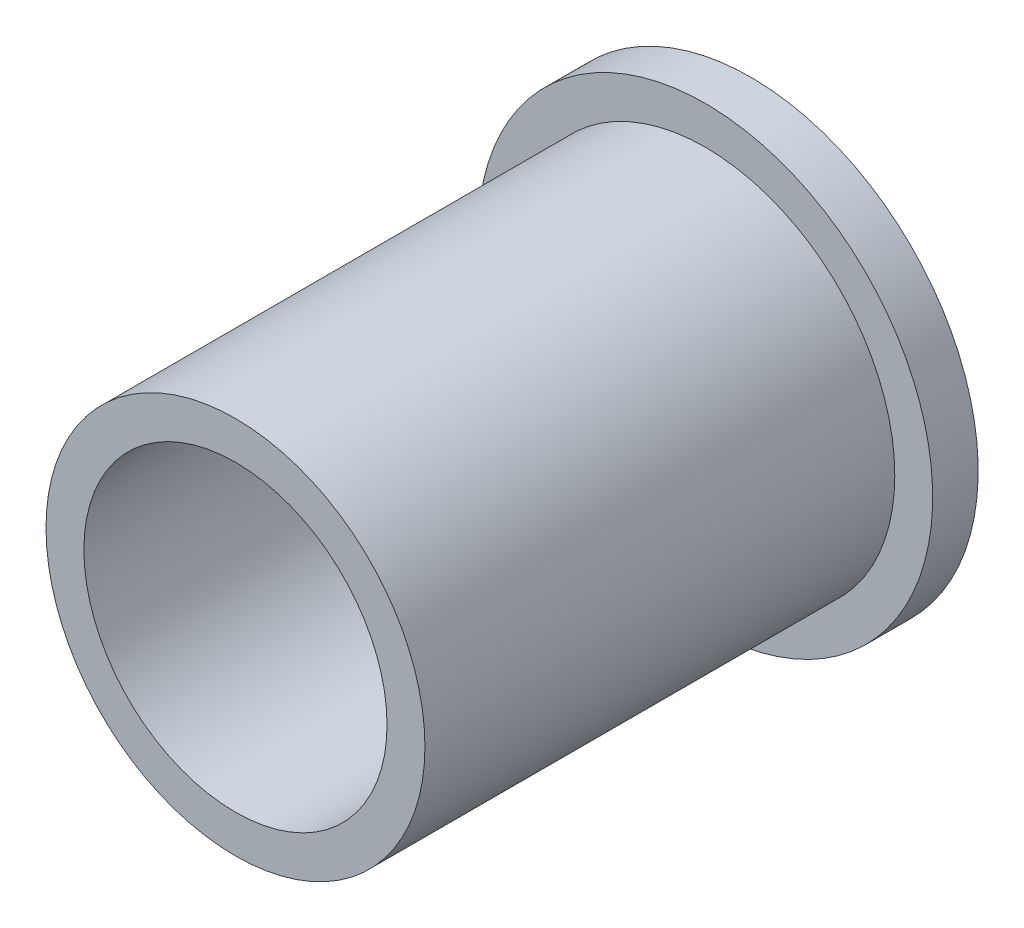
ISO-10303-21;
HEADER;
FILE_DESCRIPTION(('STEP AP214'),'2;1');
FILE_NAME('part.step','',(''),(''),'','','');
FILE_SCHEMA(('AUTOMOTIVE_DESIGN { 1 0 10303 214 1 1 1 1 }'));
ENDSEC;
DATA;
#1=APPLICATION_CONTEXT('core data for automotive mechanical design processes');
#2=APPLICATION_PROTOCOL_DEFINITION('international standard','automotive_design',2000,#1);
#3=PRODUCT_CONTEXT('',#1,'mechanical');
#4=PRODUCT('Part','Part','',(#3));
#5=PRODUCT_RELATED_PRODUCT_CATEGORY('part','',(#4));
#6=PRODUCT_DEFINITION_FORMATION('','',#4);
#7=PRODUCT_DEFINITION_CONTEXT('part definition',#1,'design');
#8=PRODUCT_DEFINITION('design','',#6,#7);
#9=PRODUCT_DEFINITION_SHAPE('','',#8);
#10=(LENGTH_UNIT() NAMED_UNIT(*) SI_UNIT(.MILLI.,.METRE.));
#11=(NAMED_UNIT(*) PLANE_ANGLE_UNIT() SI_UNIT($,.RADIAN.));
#12=(NAMED_UNIT(*) SI_UNIT($,.STERADIAN.) SOLID_ANGLE_UNIT());
#13=UNCERTAINTY_MEASURE_WITH_UNIT(LENGTH_MEASURE(1.E-05),#10,'distance_accuracy_value','');
#14=(GEOMETRIC_REPRESENTATION_CONTEXT(3) GLOBAL_UNCERTAINTY_ASSIGNED_CONTEXT((#13)) GLOBAL_UNIT_ASSIGNED_CONTEXT((#10,
#11,#12)) REPRESENTATION_CONTEXT('',''));
#15=CARTESIAN_POINT('',(0.,0.,0.));
#16=DIRECTION('',(0.,0.,1.));
#17=DIRECTION('',(1.,0.,0.));
#18=AXIS2_PLACEMENT_3D('',#15,#16,#17);
#19=CARTESIAN_POINT('',(0.,0.,31.));
#20=DIRECTION('',(0.,0.,-1.));
#21=DIRECTION('',(-1.,0.,0.));
#22=AXIS2_PLACEMENT_3D('',#19,#20,#21);
#23=CYLINDRICAL_SURFACE('',#22,12.5);
#24=CARTESIAN_POINT('',(0.,0.,31.));
#25=DIRECTION('',(0.,0.,1.));
#26=DIRECTION('',(1.,0.,0.));
#27=AXIS2_PLACEMENT_3D('',#24,#25,#26);
#28=CIRCLE('',#27,12.5);
#29=CARTESIAN_POINT('',(12.5,0.,31.));
#30=VERTEX_POINT('',#29);
#31=EDGE_CURVE('E10',#30,#30,#28,.T.);
#32=ORIENTED_EDGE('',*,*,#31,.F.);
#33=EDGE_LOOP('',(#32));
#34=FACE_BOUND('',#33,.T.);
#35=CARTESIAN_POINT('',(0.,0.,0.));
#36=DIRECTION('',(0.,0.,1.));
#37=DIRECTION('',(1.,0.,0.));
#38=AXIS2_PLACEMENT_3D('',#35,#36,#37);
#39=CIRCLE('',#38,12.5);
#40=CARTESIAN_POINT('',(12.5,0.,0.));
#41=VERTEX_POINT('',#40);
#42=EDGE_CURVE('E49',#41,#41,#39,.T.);
#43=ORIENTED_EDGE('',*,*,#42,.T.);
#44=EDGE_LOOP('',(#43));
#45=FACE_BOUND('',#44,.T.);
#46=ADVANCED_FACE('F43',(#34,#45),#23,.T.);
#47=CARTESIAN_POINT('',(0.,0.,31.));
#48=DIRECTION('',(0.,0.,1.));
#49=DIRECTION('',(1.,0.,0.));
#50=AXIS2_PLACEMENT_3D('',#47,#48,#49);
#51=PLANE('',#50);
#52=CARTESIAN_POINT('',(0.,0.,31.));
#53=DIRECTION('',(0.,0.,-1.));
#54=DIRECTION('',(-1.,0.,0.));
#55=AXIS2_PLACEMENT_3D('',#52,#53,#54);
#56=CIRCLE('',#55,10.);
#57=CARTESIAN_POINT('',(-10.,0.,31.));
#58=VERTEX_POINT('',#57);
#59=EDGE_CURVE('E65',#58,#58,#56,.T.);
#60=ORIENTED_EDGE('',*,*,#59,.T.);
#61=EDGE_LOOP('',(#60));
#62=FACE_BOUND('',#61,.T.);
#63=ORIENTED_EDGE('',*,*,#31,.T.);
#64=EDGE_LOOP('',(#63));
#65=FACE_BOUND('',#64,.T.);
#66=ADVANCED_FACE('F85',(#62,#65),#51,.T.);
#67=CARTESIAN_POINT('',(0.,0.,-3.));
#68=DIRECTION('',(0.,0.,1.));
#69=DIRECTION('',(1.,0.,0.));
#70=AXIS2_PLACEMENT_3D('',#67,#68,#69);
#71=CYLINDRICAL_SURFACE('',#70,15.);
#72=CARTESIAN_POINT('',(0.,0.,-3.));
#73=DIRECTION('',(0.,0.,-1.));
#74=DIRECTION('',(-1.,0.,0.));
#75=AXIS2_PLACEMENT_3D('',#72,#73,#74);
#76=CIRCLE('',#75,15.);
#77=CARTESIAN_POINT('',(-15.,0.,-3.));
#78=VERTEX_POINT('',#77);
#79=EDGE_CURVE('E54',#78,#78,#76,.T.);
#80=ORIENTED_EDGE('',*,*,#79,.F.);
#81=EDGE_LOOP('',(#80));
#82=FACE_BOUND('',#81,.T.);
#83=CARTESIAN_POINT('',(0.,0.,0.));
#84=DIRECTION('',(0.,0.,-1.));
#85=DIRECTION('',(-1.,0.,0.));
#86=AXIS2_PLACEMENT_3D('',#83,#84,#85);
#87=CIRCLE('',#86,15.);
#88=CARTESIAN_POINT('',(-15.,0.,0.));
#89=VERTEX_POINT('',#88);
#90=EDGE_CURVE('E60',#89,#89,#87,.T.);
#91=ORIENTED_EDGE('',*,*,#90,.T.);
#92=EDGE_LOOP('',(#91));
#93=FACE_BOUND('',#92,.T.);
#94=ADVANCED_FACE('F77',(#82,#93),#71,.T.);
#95=CARTESIAN_POINT('',(0.,0.,-3.));
#96=DIRECTION('',(0.,0.,-1.));
#97=DIRECTION('',(-1.,0.,0.));
#98=AXIS2_PLACEMENT_3D('',#95,#96,#97);
#99=PLANE('',#98);
#100=CARTESIAN_POINT('',(0.,0.,-3.));
#101=DIRECTION('',(0.,0.,-1.));
#102=DIRECTION('',(-1.,0.,0.));
#103=AXIS2_PLACEMENT_3D('',#100,#101,#102);
#104=CIRCLE('',#103,10.);
#105=CARTESIAN_POINT('',(-10.,0.,-3.));
#106=VERTEX_POINT('',#105);
#107=EDGE_CURVE('E46',#106,#106,#104,.T.);
#108=ORIENTED_EDGE('',*,*,#107,.F.);
#109=EDGE_LOOP('',(#108));
#110=FACE_BOUND('',#109,.T.);
#111=ORIENTED_EDGE('',*,*,#79,.T.);
#112=EDGE_LOOP('',(#111));
#113=FACE_BOUND('',#112,.T.);
#114=ADVANCED_FACE('F75',(#110,#113),#99,.T.);
#115=CARTESIAN_POINT('',(0.,0.,0.));
#116=DIRECTION('',(0.,0.,-1.));
#117=DIRECTION('',(-1.,0.,0.));
#118=AXIS2_PLACEMENT_3D('',#115,#116,#117);
#119=PLANE('',#118);
#120=ORIENTED_EDGE('',*,*,#42,.F.);
#121=EDGE_LOOP('',(#120));
#122=FACE_BOUND('',#121,.T.);
#123=ORIENTED_EDGE('',*,*,#90,.F.);
#124=EDGE_LOOP('',(#123));
#125=FACE_BOUND('',#124,.T.);
#126=ADVANCED_FACE('F74',(#122,#125),#119,.F.);
#127=CARTESIAN_POINT('',(0.,0.,31.));
#128=DIRECTION('',(0.,0.,-1.));
#129=DIRECTION('',(-1.,0.,0.));
#130=AXIS2_PLACEMENT_3D('',#127,#128,#129);
#131=CYLINDRICAL_SURFACE('',#130,10.);
#132=ORIENTED_EDGE('',*,*,#107,.T.);
#133=EDGE_LOOP('',(#132));
#134=FACE_BOUND('',#133,.T.);
#135=ORIENTED_EDGE('',*,*,#59,.F.);
#136=EDGE_LOOP('',(#135));
#137=FACE_BOUND('',#136,.T.);
#138=ADVANCED_FACE('F70',(#134,#137),#131,.F.);
#139=CLOSED_SHELL('',(#46,#66,#94,#114,#126,#138));
#140=MANIFOLD_SOLID_BREP('B2',#139);
#141=ADVANCED_BREP_SHAPE_REPRESENTATION('',(#18,#140),#14);
#142=SHAPE_DEFINITION_REPRESENTATION(#9,#141);
ENDSEC;
END-ISO-10303-21;
